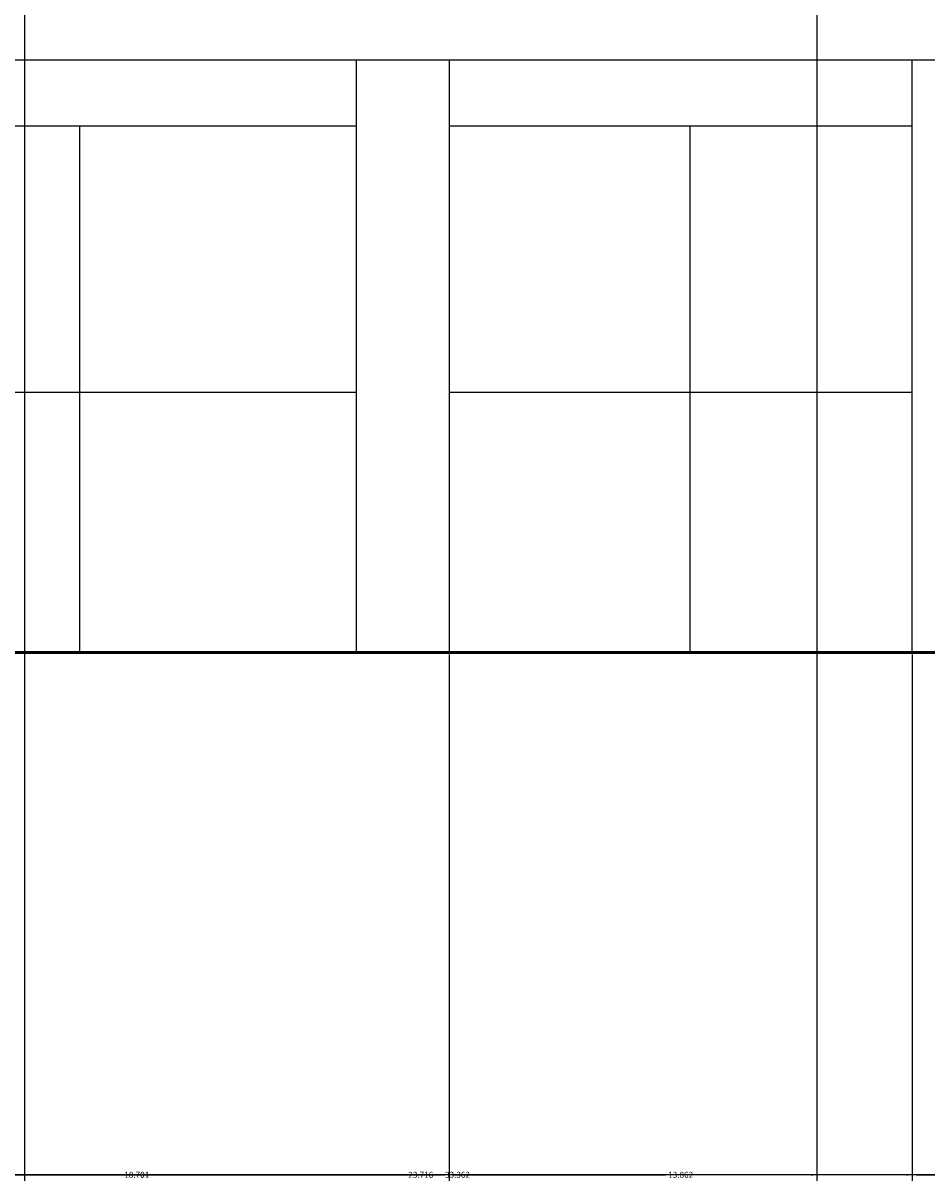
# Model space of a CAD drawing. Units: inches. Extents: x -117 to 121, y -77 to 40.
# Tile 23 of 45: x 28 to 55, y -77 to -43. Entities that reach past the tile are written whole.
import ezdxf

# ---------------------------------------------------------------- set-up
doc = ezdxf.new("R2010")
doc.units = ezdxf.units.IN
doc.header["$MEASUREMENT"] = 0
for name, color, linetype, lineweight in [('A-ANNO-DIMS', 2, 'Continuous', 18), ('A-ELEV', 7, 'Continuous', 25), ('A-ELEV-GRND', 7, 'Continuous', 50)]:
    doc.layers.add(name, color=color, linetype=linetype, lineweight=lineweight)
doc.styles.get("Standard").update_dxf_attribs({"font": 'arial.ttf'})
doc.dimstyles.get("Standard").update_dxf_attribs({"dimtxt": 0.18, "dimasz": 0.18, "dimexe": 0.18, "dimexo": 0.0625, "dimgap": 0.09, "dimtad": 0, "dimtih": 1, "dimtoh": 1, "dimdec": 4, "dimzin": 0, "dimdsep": 46, "dimtxsty": 'Standard', "dimcen": 0.09, "dimadec": 0, "dimazin": 0, "dimtfac": 1, "dimtdec": 4, "dimtofl": 0, "dimtmove": 0, "dimatfit": 3, "dimfxl": 1, "dimtolj": 1, "dimtzin": 0, "dimarcsym": 0})

# ---------------------------------------------------------------- blocks, each defined once
blk = doc.blocks.new('*D7')
at = {"layer": 'A-ANNO-DIMS', "color": 0, "lineweight": -2, "transparency": 16777216}
for p, q in [((-77.763, -61.431), (-77.763, -77.193)), ((90.549, -61.438), (90.549, -77.193)), ((-77.583, -77.013), (6.008, -77.013)), ((90.369, -77.013), (6.778, -77.013))]:
    blk.add_line(p, q, dxfattribs=at)
at = {"layer": 'A-ANNO-DIMS', "color": 0, "transparency": 16777216}
for points in [[(-77.583, -76.983), (-77.583, -77.043), (-77.763, -77.013)], [(90.369, -76.983), (90.369, -77.043), (90.549, -77.013)]]:
    blk.add_solid(points, dxfattribs=at)
at = {"layer": 'Defpoints', "color": 0, "transparency": 16777216}
for p in [(-77.763, -61.369), (90.549, -61.376), (90.549, -77.013)]:
    blk.add_point(p, dxfattribs=at)
at = {"layer": 'A-ANNO-DIMS', "color": 0, "transparency": 16777216, "insert": (6.393, -77.013), "char_height": 0.18, "attachment_point": 5}
blk.add_mtext('\\A1;168.3', dxfattribs=at)
blk = doc.blocks.new('*D26')
at = {"layer": 'A-ANNO-DIMS', "color": 0, "lineweight": -2, "transparency": 16777216}
for p, q in [((21.98, -61.438), (21.98, -77.193)), ((40.68, -61.438), (40.68, -77.193)), ((22.16, -77.013), (30.892, -77.013)), ((40.5, -77.013), (31.768, -77.013))]:
    blk.add_line(p, q, dxfattribs=at)
at = {"layer": 'A-ANNO-DIMS', "color": 0, "transparency": 16777216}
for points in [[(22.16, -76.983), (22.16, -77.043), (21.98, -77.013)], [(40.5, -76.983), (40.5, -77.043), (40.68, -77.013)]]:
    blk.add_solid(points, dxfattribs=at)
at = {"layer": 'Defpoints', "color": 0, "transparency": 16777216}
for p in [(21.98, -61.376), (40.68, -61.376), (40.68, -77.013)]:
    blk.add_point(p, dxfattribs=at)
at = {"layer": 'A-ANNO-DIMS', "color": 0, "transparency": 16777216, "insert": (31.33, -77.013), "char_height": 0.18, "attachment_point": 5}
blk.add_mtext('\\A1;18.701', dxfattribs=at)
blk = doc.blocks.new('*D27')
at = {"layer": 'A-ANNO-DIMS', "color": 0, "lineweight": -2, "transparency": 16777216}
for p, q in [((40.68, -61.438), (40.68, -77.193)), ((54.542, -61.438), (54.542, -77.193)), ((40.86, -77.013), (47.157, -77.013)), ((54.362, -77.013), (48.065, -77.013))]:
    blk.add_line(p, q, dxfattribs=at)
at = {"layer": 'A-ANNO-DIMS', "color": 0, "transparency": 16777216}
for points in [[(40.86, -76.983), (40.86, -77.043), (40.68, -77.013)], [(54.362, -76.983), (54.362, -77.043), (54.542, -77.013)]]:
    blk.add_solid(points, dxfattribs=at)
at = {"layer": 'Defpoints', "color": 0, "transparency": 16777216}
for p in [(40.68, -61.376), (54.542, -61.376), (54.542, -77.013)]:
    blk.add_point(p, dxfattribs=at)
at = {"layer": 'A-ANNO-DIMS', "color": 0, "transparency": 16777216, "insert": (47.611, -77.013), "char_height": 0.18, "attachment_point": 5}
blk.add_mtext('\\A1;13.862', dxfattribs=at)
blk = doc.blocks.new('*D28')
at = {"layer": 'A-ANNO-DIMS', "color": 0, "lineweight": -2, "transparency": 16777216}
for p, q in [((54.542, -61.438), (54.542, -77.193)), ((71.979, -61.438), (71.979, -77.193)), ((54.722, -77.013), (62.805, -77.013)), ((71.799, -77.013), (63.716, -77.013))]:
    blk.add_line(p, q, dxfattribs=at)
at = {"layer": 'A-ANNO-DIMS', "color": 0, "transparency": 16777216}
for points in [[(54.722, -76.983), (54.722, -77.043), (54.542, -77.013)], [(71.799, -76.983), (71.799, -77.043), (71.979, -77.013)]]:
    blk.add_solid(points, dxfattribs=at)
at = {"layer": 'Defpoints', "color": 0, "transparency": 16777216}
for p in [(54.542, -61.376), (71.979, -61.376), (71.979, -77.013)]:
    blk.add_point(p, dxfattribs=at)
at = {"layer": 'A-ANNO-DIMS', "color": 0, "transparency": 16777216, "insert": (63.261, -77.013), "char_height": 0.18, "attachment_point": 5}
blk.add_mtext('\\A1;17.437', dxfattribs=at)
blk = doc.blocks.new('*D53')
at = {"layer": 'A-ANNO-DIMS', "color": 0, "lineweight": -2, "transparency": 16777216}
for p, q in [((27.974, 10.841), (27.974, -77.193)), ((51.69, 10.9), (51.69, -77.193)), ((28.154, -77.013), (39.367, -77.013)), ((51.51, -77.013), (40.297, -77.013))]:
    blk.add_line(p, q, dxfattribs=at)
at = {"layer": 'A-ANNO-DIMS', "color": 0, "transparency": 16777216}
for points in [[(28.154, -76.983), (28.154, -77.043), (27.974, -77.013)], [(51.51, -76.983), (51.51, -77.043), (51.69, -77.013)]]:
    blk.add_solid(points, dxfattribs=at)
at = {"layer": 'Defpoints', "color": 0, "transparency": 16777216}
for p in [(27.974, 10.903), (51.69, 10.962), (51.69, -77.013)]:
    blk.add_point(p, dxfattribs=at)
at = {"layer": 'A-ANNO-DIMS', "color": 0, "transparency": 16777216, "insert": (39.832, -77.013), "char_height": 0.18, "attachment_point": 5}
blk.add_mtext('\\A1;23.716', dxfattribs=at)
blk = doc.blocks.new('*D58')
at = {"layer": 'A-ANNO-DIMS', "color": 0, "lineweight": -2, "transparency": 16777216}
for p, q in [((57.61, -7.947), (57.61, -77.193)), ((24.248, -8.105), (24.248, -77.193)), ((24.428, -77.013), (40.467, -77.013)), ((57.43, -77.013), (41.392, -77.013))]:
    blk.add_line(p, q, dxfattribs=at)
at = {"layer": 'A-ANNO-DIMS', "color": 0, "transparency": 16777216}
for points in [[(24.428, -76.983), (24.428, -77.043), (24.248, -77.013)], [(57.43, -76.983), (57.43, -77.043), (57.61, -77.013)]]:
    blk.add_solid(points, dxfattribs=at)
at = {"layer": 'Defpoints', "color": 0, "transparency": 16777216}
for p in [(57.61, -7.885), (24.248, -8.042), (57.61, -77.013)]:
    blk.add_point(p, dxfattribs=at)
at = {"layer": 'A-ANNO-DIMS', "color": 0, "transparency": 16777216, "insert": (40.929, -77.013), "char_height": 0.18, "attachment_point": 5}
blk.add_mtext('\\A1;33.362', dxfattribs=at)

msp = doc.modelspace()

# ---------------------------------------------------------------- linework, layer by layer
at = {"layer": 'A-ELEV'}
for p, q in [((21.9795, -43.6334), (57.4328, -43.6334)), ((37.9123, -61.3756), (37.9123, -43.6334)), ((40.6802, -43.6334), (40.6802, -61.3756)), ((54.5419, -61.3756), (54.5419, -43.6334)), ((21.9795, -45.6125), (37.9123, -45.6125)), ((29.6238, -61.3756), (29.6238, -45.6125)), ((40.6802, -45.6125), (54.5419, -45.6125)), ((47.8908, -61.3756), (47.8908, -45.6125)), ((21.9795, -53.5899), (37.9123, -53.5899)), ((40.6802, -53.5899), (54.5419, -53.5899))]:
    msp.add_line(p, q, dxfattribs=at)
at = {"layer": 'A-ELEV-GRND'}
msp.add_line((90.5486, -61.3756), (-87.9273, -61.3756), dxfattribs=at)

# ---------------------------------------------------------------- dimensions: what is measured, and where the dimension line sits
at = {"layer": 'A-ANNO-DIMS'}
for base, p1, p2, override, picture, middle in [((51.6901, -77.0135), (27.9744, 10.9032), (51.6901, 10.9623), {"dimdec": 3, "dimlfac": 1, "dimrnd": 0, "dimzin": 0, "dimdsep": 46, "dimlunit": 2}, '*D53', (39.8322, -77.0135)), ((57.6104, -77.0135), (24.2481, -8.0421), (57.6104, -7.8846), {"dimdec": 3, "dimlfac": 1, "dimrnd": 0, "dimzin": 0, "dimdsep": 46, "dimlunit": 2}, '*D58', (40.9293, -77.0135)), ((90.5486, -77.0135), (-77.7631, -61.3689), (90.5486, -61.3756), {"dimdec": 1, "dimlfac": 1, "dimrnd": 0, "dimzin": 0, "dimdsep": 46, "dimlunit": 2}, '*D7', (6.3928, -77.0135)), ((40.6802, -77.0135), (21.9795, -61.3756), (40.6802, -61.3756), {"dimdec": 3, "dimlfac": 1, "dimrnd": 0, "dimzin": 0, "dimdsep": 46, "dimlunit": 2}, '*D26', (31.3299, -77.0135)), ((54.5419, -77.0135), (40.6802, -61.3756), (54.5419, -61.3756), {"dimdec": 3, "dimlfac": 1, "dimrnd": 0, "dimzin": 0, "dimdsep": 46, "dimlunit": 2}, '*D27', (47.6111, -77.0135)), ((71.9791, -77.0135), (54.5419, -61.3756), (71.9791, -61.3756), {"dimdec": 3, "dimlfac": 1, "dimrnd": 0, "dimzin": 0, "dimdsep": 46, "dimlunit": 2}, '*D28', (63.2605, -77.0135))]:
    dim = msp.add_linear_dim(base=base, p1=p1, p2=p2, dimstyle='Standard', override=override, dxfattribs=at)
    dim.commit()
    dim.dimension.update_dxf_attribs({"geometry": picture, "text_midpoint": middle})

doc.saveas('drawing.dxf')
